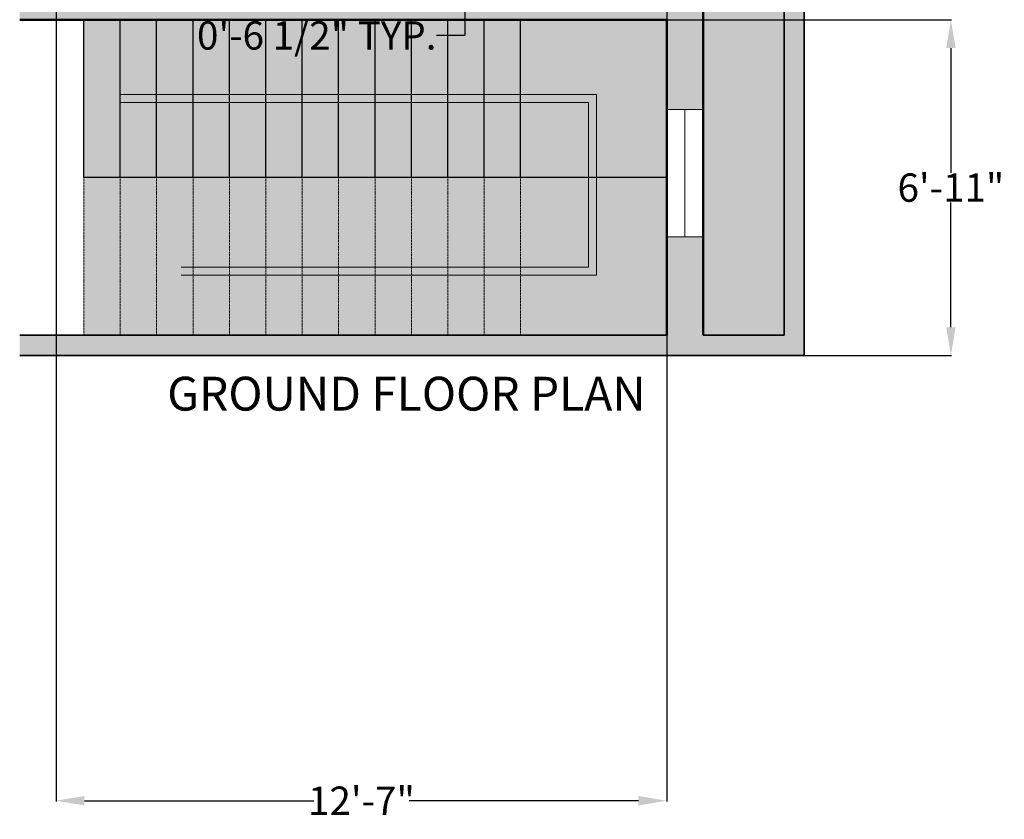
# Model space of a CAD drawing. Units: inches. Extents: x 319 to 870, y 210 to 995.
# Tile 2 of 6: x 598 to 841, y 210 to 408. Entities that reach past the tile are written whole.
import ezdxf

# ---------------------------------------------------------------- set-up
doc = ezdxf.new("R2010")
doc.units = ezdxf.units.IN
doc.header["$MEASUREMENT"] = 0
doc.linetypes.add('DASHED2', pattern=[0.375, 0.25, -0.125])
for name, color, linetype, lineweight in [('A-ANNO-DIMS', 2, 'Continuous', 18), ('A-ANNO-TITL', 7, 'Continuous', 35), ('A-FLOR-STRS', 7, 'Continuous', 25), ('A-FLOR-STRS-OVHD', 8, 'DASHED2', 18), ('A-GLAZ', 4, 'Continuous', 18), ('A-WALL', 7, 'Continuous', 50), ('A-WALL-PATT', 8, 'Continuous', 13), ('C-PROP', 7, 'Continuous', 35), ('C-PROP-PATT', 8, 'Continuous', 13)]:
    doc.layers.add(name, color=color, linetype=linetype, lineweight=lineweight)
for name, color, linetype, lineweight, true_color in [('A-ANNO-STRS', 16, 'Continuous', 18, 0x6c0707), ('A-ANNO-SYMB-PATT', 16, 'Continuous', 13, 0x6c0707), ('A-FLOR-STRS-PATT', 144, 'Continuous', 13, 0x1e788f), ('C-SITE-PATT', 126, 'Continuous', 13, 0x1e6f63)]:
    doc.layers.add(name, color=color, linetype=linetype, lineweight=lineweight, true_color=true_color)
doc.styles.get("Standard").update_dxf_attribs({"font": 'arial.ttf'})
doc.dimstyles.get("Standard").update_dxf_attribs({"dimtxt": 7, "dimasz": 7, "dimexe": 0.18, "dimexo": 0.0625, "dimgap": 0.09, "dimtad": 0, "dimtih": 1, "dimtoh": 1, "dimdec": 0, "dimzin": 0, "dimdsep": 46, "dimlunit": 3, "dimtxsty": 'Standard', "dimcen": 0.09, "dimadec": 0, "dimazin": 0, "dimtfac": 1, "dimtdec": 0, "dimtofl": 0, "dimtmove": 0, "dimatfit": 3, "dimfxl": 1, "dimtolj": 1, "dimtzin": 0, "dimarcsym": 0})

# ---------------------------------------------------------------- blocks, each defined once
blk = doc.blocks.new('Moment Connection - Imperial')
at = {"color": 0}
blk.add_solid([(0, 0.125), (0.125, 0.0625), (0, 0)], dxfattribs=at)
blk = doc.blocks.new('*D39')
at = {"layer": 'A-ANNO-DIMS', "color": 0, "lineweight": -2, "transparency": 16777216}
for p, q in [((696.21, 417.72), (696.21, 416.1)), ((706.21, 417.72), (706.21, 416.1)), ((689.21, 416.28), (682.21, 416.28)), ((713.21, 416.28), (720.21, 416.28))]:
    blk.add_line(p, q, dxfattribs=at)
at = {"layer": 'A-ANNO-DIMS', "color": 0, "transparency": 16777216}
for points in [[(689.21, 417.45), (689.21, 415.11), (696.21, 416.28)], [(713.21, 417.45), (713.21, 415.11), (706.21, 416.28)]]:
    blk.add_solid(points, dxfattribs=at)
at = {"layer": 'Defpoints', "color": 0, "transparency": 16777216}
for p in [(696.21, 417.78), (706.21, 417.78), (696.21, 416.28)]:
    blk.add_point(p, dxfattribs=at)
at = {"layer": 'A-ANNO-DIMS', "color": 0, "transparency": 16777216, "insert": (632.95, 416.28), "char_height": 7, "attachment_point": 5}
blk.add_mtext('\\A1;BATH TAP 0\'-10" TYP.', dxfattribs=at)
blk = doc.blocks.new('*D40')
at = {"layer": 'A-ANNO-DIMS', "color": 0, "lineweight": -2, "transparency": 16777216}
for p, q in [((707.71, 431.28), (707.71, 438.28)), ((706.27, 424.28), (707.89, 424.28)), ((706.27, 417.78), (707.89, 417.78)), ((707.71, 410.78), (707.71, 403.78)), ((707.71, 403.78), (700.71, 403.78))]:
    blk.add_line(p, q, dxfattribs=at)
at = {"layer": 'A-ANNO-DIMS', "color": 0, "transparency": 16777216}
for points in [[(706.54, 431.28), (708.87, 431.28), (707.71, 424.28)], [(706.54, 410.78), (708.87, 410.78), (707.71, 417.78)]]:
    blk.add_solid(points, dxfattribs=at)
at = {"layer": 'Defpoints', "color": 0, "transparency": 16777216}
for p in [(706.21, 424.28), (706.21, 417.78), (707.71, 417.78)]:
    blk.add_point(p, dxfattribs=at)
at = {"layer": 'A-ANNO-DIMS', "color": 0, "transparency": 16777216, "insert": (671.13, 403.78), "char_height": 7, "attachment_point": 5}
blk.add_mtext('\\A1;0\'-6 1/2" TYP.', dxfattribs=at)
blk = doc.blocks.new('*D51')
at = {"layer": 'A-ANNO-DIMS', "color": 0, "lineweight": -2, "transparency": 16777216}
for p, q in [((757.75, 407.67), (828.11, 407.67)), ((827.93, 400.67), (827.93, 369.83)), ((827.93, 331.67), (827.93, 362.5)), ((791.75, 324.67), (828.11, 324.67))]:
    blk.add_line(p, q, dxfattribs=at)
at = {"layer": 'A-ANNO-DIMS', "color": 0, "transparency": 16777216}
for points in [[(826.77, 400.67), (829.1, 400.67), (827.93, 407.67)], [(826.77, 331.67), (829.1, 331.67), (827.93, 324.67)]]:
    blk.add_solid(points, dxfattribs=at)
at = {"layer": 'Defpoints', "color": 0, "transparency": 16777216}
for p in [(757.68, 407.67), (827.93, 407.67), (791.68, 324.67)]:
    blk.add_point(p, dxfattribs=at)
at = {"layer": 'A-ANNO-DIMS', "color": 0, "transparency": 16777216, "insert": (827.93, 366.17), "char_height": 7, "attachment_point": 5}
blk.add_mtext('\\A1;6\'-11"', dxfattribs=at)
blk = doc.blocks.new('*D53')
at = {"layer": 'A-ANNO-DIMS', "color": 0, "lineweight": -2, "transparency": 16777216}
for p, q in [((606.68, 416.61), (606.68, 214.45)), ((757.68, 416.61), (757.68, 214.45)), ((613.68, 214.63), (670.4, 214.63)), ((750.68, 214.63), (693.97, 214.63))]:
    blk.add_line(p, q, dxfattribs=at)
at = {"layer": 'A-ANNO-DIMS', "color": 0, "transparency": 16777216}
for points in [[(613.68, 215.8), (613.68, 213.47), (606.68, 214.63)], [(750.68, 215.8), (750.68, 213.47), (757.68, 214.63)]]:
    blk.add_solid(points, dxfattribs=at)
at = {"layer": 'Defpoints', "color": 0, "transparency": 16777216}
for p in [(606.68, 416.67), (757.68, 416.67), (757.68, 214.63)]:
    blk.add_point(p, dxfattribs=at)
at = {"layer": 'A-ANNO-DIMS', "color": 0, "transparency": 16777216, "insert": (682.18, 214.63), "char_height": 7, "attachment_point": 5}
blk.add_mtext('\\A1;12\'-7"', dxfattribs=at)

msp = doc.modelspace()

# ---------------------------------------------------------------- hatches: boundary and pattern name
at = {"layer": 'A-ANNO-SYMB-PATT'}
h = msp.add_hatch(color=256, dxfattribs=at)
h.dxf.hatch_style = 1
h.paths.add_polyline_path([(631.54, 387.17), (631.54, 389.17), (622.54, 389.17), (622.54, 387.17)])
h = msp.add_hatch(color=256, dxfattribs=at)
h.dxf.hatch_style = 1
h.paths.add_polyline_path([(640.54, 387.17), (640.54, 389.17), (631.54, 389.17), (631.54, 387.17)])
h = msp.add_hatch(color=256, dxfattribs=at)
h.dxf.hatch_style = 1
h.paths.add_polyline_path([(640.54, 389.17), (640.54, 387.17), (649.54, 387.17), (649.54, 389.17)])
h = msp.add_hatch(color=256, dxfattribs=at)
h.dxf.hatch_style = 1
h.paths.add_polyline_path([(658.54, 387.17), (658.54, 389.17), (649.54, 389.17), (649.54, 387.17)])
h = msp.add_hatch(color=256, dxfattribs=at)
h.dxf.hatch_style = 1
h.paths.add_polyline_path([(658.54, 389.17), (658.54, 387.17), (667.54, 387.17), (667.54, 389.17)])
h = msp.add_hatch(color=256, dxfattribs=at)
h.dxf.hatch_style = 1
h.paths.add_polyline_path([(676.54, 387.17), (676.54, 389.17), (667.54, 389.17), (667.54, 387.17)])
h = msp.add_hatch(color=256, dxfattribs=at)
h.dxf.hatch_style = 1
h.paths.add_polyline_path([(676.54, 389.17), (676.54, 387.17), (685.54, 387.17), (685.54, 389.17)])
h = msp.add_hatch(color=256, dxfattribs=at)
h.dxf.hatch_style = 1
h.paths.add_polyline_path([(685.54, 389.17), (685.54, 387.17), (694.54, 387.17), (694.54, 389.17)])
h = msp.add_hatch(color=256, dxfattribs=at)
h.dxf.hatch_style = 1
h.paths.add_polyline_path([(694.54, 389.17), (694.54, 387.17), (703.54, 387.17), (703.54, 389.17)])
h = msp.add_hatch(color=256, dxfattribs=at)
h.dxf.hatch_style = 1
h.paths.add_polyline_path([(703.54, 389.17), (703.54, 387.17), (712.54, 387.17), (712.54, 389.17)])
h = msp.add_hatch(color=256, dxfattribs=at)
h.dxf.hatch_style = 1
h.paths.add_polyline_path([(712.54, 389.17), (712.54, 387.17), (721.54, 387.17), (721.54, 389.17)])
h = msp.add_hatch(color=256, dxfattribs=at)
h.dxf.hatch_style = 1
h.paths.add_polyline_path([(740.32, 389.17), (721.54, 389.17), (721.54, 387.17), (738.32, 387.17), (738.32, 368.67), (740.32, 368.67)])
h = msp.add_hatch(color=256, dxfattribs=at)
h.dxf.hatch_style = 1
h.paths.add_polyline_path([(740.32, 344.52), (740.32, 368.67), (738.32, 368.67), (738.32, 346.52), (721.54, 346.52), (721.54, 344.52)])
h = msp.add_hatch(color=256, dxfattribs=at)
h.dxf.hatch_style = 1
h.paths.add_polyline_path([(649.54, 344.52), (649.54, 346.52), (640.54, 346.52), (640.54, 344.52)])
h = msp.add_hatch(color=256, dxfattribs=at)
h.dxf.hatch_style = 1
h.paths.add_polyline_path([(658.54, 344.52), (658.54, 346.52), (649.54, 346.52), (649.54, 344.52)])
h = msp.add_hatch(color=256, dxfattribs=at)
h.dxf.hatch_style = 1
h.paths.add_polyline_path([(667.54, 344.52), (667.54, 346.52), (658.54, 346.52), (658.54, 344.52)])
h = msp.add_hatch(color=256, dxfattribs=at)
h.dxf.hatch_style = 1
h.paths.add_polyline_path([(676.54, 344.52), (676.54, 346.52), (667.54, 346.52), (667.54, 344.52)])
h = msp.add_hatch(color=256, dxfattribs=at)
h.dxf.hatch_style = 1
h.paths.add_polyline_path([(685.54, 344.52), (685.54, 346.52), (676.54, 346.52), (676.54, 344.52)])
h = msp.add_hatch(color=256, dxfattribs=at)
h.dxf.hatch_style = 1
h.paths.add_polyline_path([(694.54, 344.52), (694.54, 346.52), (685.54, 346.52), (685.54, 344.52)])
h = msp.add_hatch(color=256, dxfattribs=at)
h.dxf.hatch_style = 1
h.paths.add_polyline_path([(703.54, 344.52), (703.54, 346.52), (694.54, 346.52), (694.54, 344.52)])
h = msp.add_hatch(color=256, dxfattribs=at)
h.dxf.hatch_style = 1
h.paths.add_polyline_path([(712.54, 344.52), (712.54, 346.52), (703.54, 346.52), (703.54, 344.52)])
h = msp.add_hatch(color=256, dxfattribs=at)
h.dxf.hatch_style = 1
h.paths.add_polyline_path([(712.54, 346.52), (712.54, 344.52), (721.54, 344.52), (721.54, 346.52)])
at = {"layer": 'A-FLOR-STRS-PATT'}
h = msp.add_hatch(color=256, dxfattribs=at)
h.dxf.hatch_style = 1
h.paths.add_polyline_path([(622.54, 407.67), (613.54, 407.67), (613.54, 368.67), (622.54, 368.67)])
h = msp.add_hatch(color=256, dxfattribs=at)
h.dxf.hatch_style = 1
h.paths.add_polyline_path([(631.54, 407.67), (622.54, 407.67), (622.54, 389.17), (631.54, 389.17)])
h = msp.add_hatch(color=256, dxfattribs=at)
h.dxf.hatch_style = 1
h.paths.add_polyline_path([(631.54, 407.67), (622.54, 407.67), (622.54, 389.17), (631.54, 389.17)])
h = msp.add_hatch(color=256, dxfattribs=at)
h.dxf.hatch_style = 1
h.paths.add_polyline_path([(640.54, 407.67), (631.54, 407.67), (631.54, 389.17), (640.54, 389.17)])
h = msp.add_hatch(color=256, dxfattribs=at)
h.dxf.hatch_style = 1
h.paths.add_polyline_path([(640.54, 389.17), (649.54, 389.17), (649.54, 407.67), (640.54, 407.67)])
h = msp.add_hatch(color=256, dxfattribs=at)
h.dxf.hatch_style = 1
h.paths.add_polyline_path([(649.54, 407.67), (640.54, 407.67), (640.54, 389.17), (649.54, 389.17)])
h = msp.add_hatch(color=256, dxfattribs=at)
h.dxf.hatch_style = 1
h.paths.add_polyline_path([(658.54, 407.67), (649.54, 407.67), (649.54, 389.17), (658.54, 389.17)])
h = msp.add_hatch(color=256, dxfattribs=at)
h.dxf.hatch_style = 1
h.paths.add_polyline_path([(667.54, 407.67), (658.54, 407.67), (658.54, 389.17), (667.54, 389.17)])
h = msp.add_hatch(color=256, dxfattribs=at)
h.dxf.hatch_style = 1
h.paths.add_polyline_path([(658.54, 389.17), (667.54, 389.17), (667.54, 407.67), (658.54, 407.67)])
h = msp.add_hatch(color=256, dxfattribs=at)
h.dxf.hatch_style = 1
h.paths.add_polyline_path([(667.54, 389.17), (676.54, 389.17), (676.54, 407.67), (667.54, 407.67)])
h = msp.add_hatch(color=256, dxfattribs=at)
h.dxf.hatch_style = 1
h.paths.add_polyline_path([(685.54, 407.67), (676.54, 407.67), (676.54, 389.17), (685.54, 389.17)])
h = msp.add_hatch(color=256, dxfattribs=at)
h.dxf.hatch_style = 1
h.paths.add_polyline_path([(685.54, 407.67), (676.54, 407.67), (676.54, 389.17), (685.54, 389.17)])
h = msp.add_hatch(color=256, dxfattribs=at)
h.dxf.hatch_style = 1
h.paths.add_polyline_path([(685.54, 389.17), (694.54, 389.17), (694.54, 407.67), (685.54, 407.67)])
h = msp.add_hatch(color=256, dxfattribs=at)
h.dxf.hatch_style = 1
h.paths.add_polyline_path([(694.54, 389.17), (703.54, 389.17), (703.54, 407.67), (694.54, 407.67)])
h = msp.add_hatch(color=256, dxfattribs=at)
h.dxf.hatch_style = 1
h.paths.add_polyline_path([(694.54, 389.17), (703.54, 389.17), (703.54, 407.67), (694.54, 407.67)])
h = msp.add_hatch(color=256, dxfattribs=at)
h.dxf.hatch_style = 1
h.paths.add_polyline_path([(712.54, 407.67), (703.54, 407.67), (703.54, 389.17), (712.54, 389.17)])
h = msp.add_hatch(color=256, dxfattribs=at)
h.dxf.hatch_style = 1
h.paths.add_polyline_path([(721.54, 407.67), (712.54, 407.67), (712.54, 389.17), (721.54, 389.17)])
h = msp.add_hatch(color=256, dxfattribs=at)
h.dxf.hatch_style = 1
h.paths.add_polyline_path([(740.32, 389.17), (740.32, 368.67), (757.68, 368.67), (757.68, 407.67), (721.54, 407.67), (721.54, 389.17)])
h = msp.add_hatch(color=256, dxfattribs=at)
h.dxf.hatch_style = 1
h.paths.add_polyline_path([(622.54, 368.67), (631.54, 368.67), (631.54, 387.17), (622.54, 387.17)])
h = msp.add_hatch(color=256, dxfattribs=at)
h.dxf.hatch_style = 1
h.paths.add_polyline_path([(622.54, 368.67), (631.54, 368.67), (631.54, 387.17), (622.54, 387.17)])
h = msp.add_hatch(color=256, dxfattribs=at)
h.dxf.hatch_style = 1
h.paths.add_polyline_path([(640.54, 387.17), (631.54, 387.17), (631.54, 368.67), (640.54, 368.67)])
h = msp.add_hatch(color=256, dxfattribs=at)
h.dxf.hatch_style = 1
h.paths.add_polyline_path([(640.54, 368.67), (649.54, 368.67), (649.54, 387.17), (640.54, 387.17)])
h = msp.add_hatch(color=256, dxfattribs=at)
h.dxf.hatch_style = 1
h.paths.add_polyline_path([(640.54, 368.67), (649.54, 368.67), (649.54, 387.17), (640.54, 387.17)])
h = msp.add_hatch(color=256, dxfattribs=at)
h.dxf.hatch_style = 1
h.paths.add_polyline_path([(658.54, 387.17), (649.54, 387.17), (649.54, 368.67), (658.54, 368.67)])
h = msp.add_hatch(color=256, dxfattribs=at)
h.dxf.hatch_style = 1
h.paths.add_polyline_path([(658.54, 368.67), (667.54, 368.67), (667.54, 387.17), (658.54, 387.17)])
h = msp.add_hatch(color=256, dxfattribs=at)
h.dxf.hatch_style = 1
h.paths.add_polyline_path([(667.54, 387.17), (658.54, 387.17), (658.54, 368.67), (667.54, 368.67)])
h = msp.add_hatch(color=256, dxfattribs=at)
h.dxf.hatch_style = 1
h.paths.add_polyline_path([(667.54, 368.67), (676.54, 368.67), (676.54, 387.17), (667.54, 387.17)])
h = msp.add_hatch(color=256, dxfattribs=at)
h.dxf.hatch_style = 1
h.paths.add_polyline_path([(676.54, 368.67), (685.54, 368.67), (685.54, 387.17), (676.54, 387.17)])
h = msp.add_hatch(color=256, dxfattribs=at)
h.dxf.hatch_style = 1
h.paths.add_polyline_path([(685.54, 387.17), (676.54, 387.17), (676.54, 368.67), (685.54, 368.67)])
h = msp.add_hatch(color=256, dxfattribs=at)
h.dxf.hatch_style = 1
h.paths.add_polyline_path([(685.54, 368.67), (694.54, 368.67), (694.54, 387.17), (685.54, 387.17)])
h = msp.add_hatch(color=256, dxfattribs=at)
h.dxf.hatch_style = 1
h.paths.add_polyline_path([(694.54, 368.67), (703.54, 368.67), (703.54, 387.17), (694.54, 387.17)])
h = msp.add_hatch(color=256, dxfattribs=at)
h.dxf.hatch_style = 1
h.paths.add_polyline_path([(694.54, 368.67), (703.54, 368.67), (703.54, 387.17), (694.54, 387.17)])
h = msp.add_hatch(color=256, dxfattribs=at)
h.dxf.hatch_style = 1
h.paths.add_polyline_path([(703.54, 368.67), (712.54, 368.67), (712.54, 387.17), (703.54, 387.17)])
h = msp.add_hatch(color=256, dxfattribs=at)
h.dxf.hatch_style = 1
h.paths.add_polyline_path([(712.54, 368.67), (721.54, 368.67), (721.54, 387.17), (712.54, 387.17)])
h = msp.add_hatch(color=256, dxfattribs=at)
h.dxf.hatch_style = 1
h.paths.add_polyline_path([(721.54, 368.67), (738.32, 368.67), (738.32, 387.17), (721.54, 387.17)])
h = msp.add_hatch(color=256, dxfattribs=at)
h.dxf.hatch_style = 1
h.paths.add_polyline_path([(622.54, 368.67), (613.54, 368.67), (613.54, 329.67), (622.54, 329.67)])
h = msp.add_hatch(color=256, dxfattribs=at)
h.dxf.hatch_style = 1
h.paths.add_polyline_path([(631.54, 368.67), (622.54, 368.67), (622.54, 329.67), (631.54, 329.67)])
h = msp.add_hatch(color=256, dxfattribs=at)
h.dxf.hatch_style = 1
h.paths.add_polyline_path([(640.54, 368.67), (631.54, 368.67), (631.54, 329.67), (640.54, 329.67)])
h = msp.add_hatch(color=256, dxfattribs=at)
h.dxf.hatch_style = 1
h.paths.add_polyline_path([(640.54, 346.52), (649.54, 346.52), (649.54, 368.67), (640.54, 368.67)])
h = msp.add_hatch(color=256, dxfattribs=at)
h.dxf.hatch_style = 1
h.paths.add_polyline_path([(658.54, 368.67), (649.54, 368.67), (649.54, 346.52), (658.54, 346.52)])
h = msp.add_hatch(color=256, dxfattribs=at)
h.dxf.hatch_style = 1
h.paths.add_polyline_path([(658.54, 346.52), (667.54, 346.52), (667.54, 368.67), (658.54, 368.67)])
h = msp.add_hatch(color=256, dxfattribs=at)
h.dxf.hatch_style = 1
h.paths.add_polyline_path([(667.54, 346.52), (676.54, 346.52), (676.54, 368.67), (667.54, 368.67)])
h = msp.add_hatch(color=256, dxfattribs=at)
h.dxf.hatch_style = 1
h.paths.add_polyline_path([(685.54, 368.67), (676.54, 368.67), (676.54, 346.52), (685.54, 346.52)])
h = msp.add_hatch(color=256, dxfattribs=at)
h.dxf.hatch_style = 1
h.paths.add_polyline_path([(694.54, 346.52), (694.54, 368.67), (685.54, 368.67), (685.54, 346.52)])
h = msp.add_hatch(color=256, dxfattribs=at)
h.dxf.hatch_style = 1
h.paths.add_polyline_path([(694.54, 346.52), (703.54, 346.52), (703.54, 368.67), (694.54, 368.67)])
h = msp.add_hatch(color=256, dxfattribs=at)
h.dxf.hatch_style = 1
h.paths.add_polyline_path([(712.54, 368.67), (703.54, 368.67), (703.54, 346.52), (712.54, 346.52)])
h = msp.add_hatch(color=256, dxfattribs=at)
h.dxf.hatch_style = 1
h.paths.add_polyline_path([(712.54, 346.52), (721.54, 346.52), (721.54, 368.67), (712.54, 368.67)])
h = msp.add_hatch(color=256, dxfattribs=at)
h.dxf.hatch_style = 1
h.paths.add_polyline_path([(738.32, 368.67), (721.54, 368.67), (721.54, 346.52), (738.32, 346.52)])
h = msp.add_hatch(color=256, dxfattribs=at)
h.dxf.hatch_style = 1
h.paths.add_polyline_path([(757.68, 368.67), (740.32, 368.67), (740.32, 344.52), (721.54, 344.52), (721.54, 329.67), (757.68, 329.67)])
h = msp.add_hatch(color=256, dxfattribs=at)
h.dxf.hatch_style = 1
h.paths.add_polyline_path([(649.54, 344.52), (640.54, 344.52), (640.54, 329.67), (649.54, 329.67)])
h = msp.add_hatch(color=256, dxfattribs=at)
h.dxf.hatch_style = 1
h.paths.add_polyline_path([(658.54, 344.52), (649.54, 344.52), (649.54, 329.67), (658.54, 329.67)])
h = msp.add_hatch(color=256, dxfattribs=at)
h.dxf.hatch_style = 1
h.paths.add_polyline_path([(667.54, 344.52), (658.54, 344.52), (658.54, 329.67), (667.54, 329.67)])
h = msp.add_hatch(color=256, dxfattribs=at)
h.dxf.hatch_style = 1
h.paths.add_polyline_path([(667.54, 329.67), (676.54, 329.67), (676.54, 344.52), (667.54, 344.52)])
h = msp.add_hatch(color=256, dxfattribs=at)
h.dxf.hatch_style = 1
h.paths.add_polyline_path([(676.54, 344.52), (676.54, 329.67), (685.54, 329.67), (685.54, 344.52)])
h = msp.add_hatch(color=256, dxfattribs=at)
h.dxf.hatch_style = 1
h.paths.add_polyline_path([(694.54, 344.52), (685.54, 344.52), (685.54, 329.67), (694.54, 329.67)])
h = msp.add_hatch(color=256, dxfattribs=at)
h.dxf.hatch_style = 1
h.paths.add_polyline_path([(694.54, 329.67), (703.54, 329.67), (703.54, 344.52), (694.54, 344.52)])
h = msp.add_hatch(color=256, dxfattribs=at)
h.dxf.hatch_style = 1
h.paths.add_polyline_path([(712.54, 344.52), (703.54, 344.52), (703.54, 329.67), (712.54, 329.67)])
h = msp.add_hatch(color=256, dxfattribs=at)
h.dxf.hatch_style = 1
h.paths.add_polyline_path([(721.54, 344.52), (712.54, 344.52), (712.54, 329.67), (721.54, 329.67)])
at = {"layer": 'A-WALL-PATT'}
h = msp.add_hatch(color=256, dxfattribs=at)
h.dxf.hatch_style = 1
h.paths.add_polyline_path([(606.68, 476.67), (628.53, 476.67), (628.53, 485.67), (606.68, 485.67), (606.68, 614.99), (597.68, 614.99), (597.68, 407.67), (757.68, 407.67), (757.68, 385.48), (766.68, 385.48), (766.68, 431.25), (757.68, 431.25), (757.68, 416.67), (606.68, 416.67)])
at = {"layer": 'C-PROP-PATT'}
h = msp.add_hatch(color=256, dxfattribs=at)
h.dxf.hatch_style = 1
h.paths.add_polyline_path([(757.68, 329.67), (597.68, 329.67), (597.68, 324.67), (791.68, 324.67), (791.68, 948.67), (376.68, 948.67), (376.68, 943.67), (786.68, 943.67), (786.68, 329.67), (766.68, 329.67), (766.68, 354.04), (757.68, 354.04)])
at = {"layer": 'C-SITE-PATT'}
h = msp.add_hatch(color=256, dxfattribs=at)
h.dxf.hatch_style = 1
h.paths.add_polyline_path([(376.68, 515.67), (396.68, 515.67), (396.68, 923.67), (528.68, 923.67), (606.68, 923.67), (766.68, 923.67), (766.68, 329.67), (786.68, 329.67), (786.68, 943.67), (376.68, 943.67)])
h.paths.add_polyline_path([(392.17, 638.98), (392.17, 682.3), (381.61, 682.3), (381.61, 638.98)], flags=24)
h.paths.add_polyline_path([(772.77, 716.95), (772.77, 673.64), (783.33, 673.64), (783.33, 716.95)], flags=24)
h.paths.add_polyline_path([(542.27, 929.56), (581.61, 929.56), (581.61, 939.15), (542.27, 939.15)], flags=24)

# ---------------------------------------------------------------- linework, layer by layer
at = {"layer": 'A-ANNO-STRS'}
for p, q in [((622.54, 389.17), (740.32, 389.17)), ((622.54, 387.17), (738.32, 387.17)), ((738.32, 387.17), (738.32, 346.52)), ((740.32, 389.17), (740.32, 344.52)), ((738.32, 346.52), (637.59, 346.52)), ((740.32, 344.52), (637.59, 344.52))]:
    msp.add_line(p, q, dxfattribs=at)
at = {"layer": 'A-FLOR-STRS'}
for p, q in [((613.54, 368.67), (613.54, 407.67)), ((622.54, 368.67), (622.54, 407.67)), ((631.54, 368.67), (631.54, 407.67)), ((640.54, 368.67), (640.54, 407.67)), ((649.54, 368.67), (649.54, 407.67)), ((658.54, 368.67), (658.54, 407.67)), ((667.54, 368.67), (667.54, 407.67)), ((676.54, 368.67), (676.54, 407.67)), ((685.54, 368.67), (685.54, 407.67)), ((694.54, 368.67), (694.54, 407.67)), ((703.54, 368.67), (703.54, 407.67)), ((712.54, 368.67), (712.54, 407.67)), ((721.54, 368.67), (721.54, 407.67)), ((757.68, 368.67), (613.54, 368.67))]:
    msp.add_line(p, q, dxfattribs=at)
at = {"layer": 'A-FLOR-STRS-OVHD'}
for p, q in [((613.54, 368.67), (613.54, 329.67)), ((622.54, 368.67), (622.54, 329.67)), ((631.54, 368.67), (631.54, 329.67)), ((640.54, 368.67), (640.54, 329.67)), ((649.54, 368.67), (649.54, 329.67)), ((658.54, 368.67), (658.54, 329.67)), ((667.54, 368.67), (667.54, 329.67)), ((676.54, 368.67), (676.54, 329.67)), ((685.54, 368.67), (685.54, 329.67)), ((694.54, 368.67), (694.54, 329.67)), ((703.54, 368.67), (703.54, 329.67)), ((712.54, 368.67), (712.54, 329.67)), ((721.54, 368.67), (721.54, 329.67))]:
    msp.add_line(p, q, dxfattribs=at)
at = {"layer": 'A-GLAZ'}
for p, q in [((757.68, 385.48), (766.68, 385.48)), ((762.18, 385.48), (762.18, 354.04)), ((757.68, 354.04), (766.68, 354.04))]:
    msp.add_line(p, q, dxfattribs=at)
at = {"layer": 'A-WALL'}
for p, q in [((766.68, 329.67), (766.68, 923.67)), ((766.68, 731.67), (766.68, 329.67)), ((757.68, 407.67), (597.68, 407.67)), ((757.68, 407.67), (757.68, 329.67))]:
    msp.add_line(p, q, dxfattribs=at)
at = {"layer": 'C-PROP'}
for p, q in [((791.68, 324.67), (791.68, 948.67)), ((786.68, 329.67), (786.68, 943.67)), ((597.68, 329.67), (757.68, 329.67)), ((766.68, 329.67), (786.68, 329.67)), ((597.68, 324.67), (791.68, 324.67))]:
    msp.add_line(p, q, dxfattribs=at)

# ---------------------------------------------------------------- block references
at = {"layer": 'A-ANNO-STRS', "xscale": 43.4388041049242, "yscale": 43.4388041049242, "zscale": 43.4388041049242, "rotation": 180}
msp.add_blockref('Moment Connection - Imperial', (637.59, 348.24), dxfattribs=at)

# ---------------------------------------------------------------- texts
at = {"layer": 'A-ANNO-TITL', "insert": (634.16, 319.42), "char_height": 8.3641, "attachment_point": 1}
msp.add_mtext_dynamic_manual_height_columns('GROUND FLOOR PLAN', width=137.9446, gutter_width=41.82, heights=[0], dxfattribs=at)

# ---------------------------------------------------------------- dimensions: what is measured, and where the dimension line sits
at = {"layer": 'A-ANNO-DIMS'}
for base, p1, p2, angle, text, picture, middle in [((696.21, 416.28), (706.21, 417.78), (696.21, 417.78), 180, 'BATH TAP <> TYP.', '*D39', (632.95, 416.28)), ((707.71, 417.78), (706.21, 424.28), (706.21, 417.78), 270, '<> TYP.', '*D40', (671.13, 403.78))]:
    dim = msp.add_linear_dim(base=base, p1=p1, p2=p2, angle=angle, text=text, dimstyle='Standard', override={"dimdec": 1, "dimlfac": 1, "dimrnd": 0, "dimzin": 1, "dimdsep": 46, "dimlunit": 4, "dimfrac": 2}, dxfattribs=at)
    dim.commit()
    dim.dimension.update_dxf_attribs({"geometry": picture, "text_midpoint": middle})
dim = msp.add_linear_dim(base=(757.68, 214.63), p1=(606.68, 416.67), p2=(757.68, 416.67), dimstyle='Standard', override={"dimdec": 1, "dimlfac": 1, "dimrnd": 0, "dimzin": 1, "dimdsep": 46, "dimlunit": 4, "dimfrac": 2}, dxfattribs=at)
dim.commit()
dim.dimension.update_dxf_attribs({"geometry": '*D53', "text_midpoint": (682.18, 214.63)})
dim = msp.add_linear_dim(base=(827.93, 407.67), p1=(791.68, 324.67), p2=(757.68, 407.67), angle=90, dimstyle='Standard', override={"dimdec": 1, "dimlfac": 1, "dimrnd": 0, "dimzin": 1, "dimdsep": 46, "dimlunit": 4, "dimfrac": 2}, dxfattribs=at)
dim.commit()
dim.dimension.update_dxf_attribs({"geometry": '*D51', "text_midpoint": (827.93, 366.17)})

doc.saveas('drawing.dxf')
